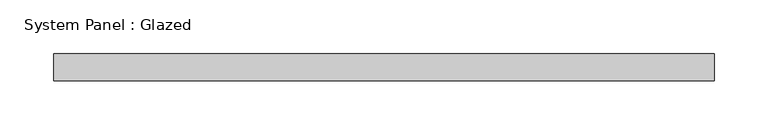
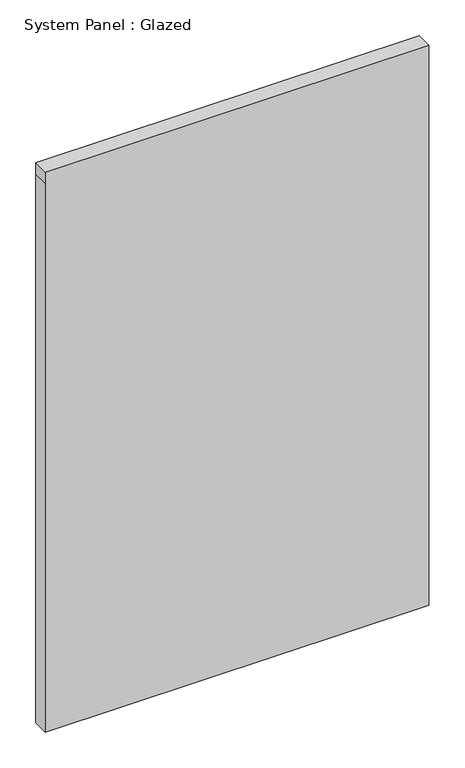
"""IFC4 building model written with IfcOpenShell, lengths in millimetres: plate geometry, System Panel : Glazed."""

from ifc_helpers import new_model, si_unit, frame, origin, place, context, project, spatial, polyline, outline, extrude, source, transform, mapped, element, save


def system_panel_glazed_bb181a04(model_context):
    return source(origin(), model_context, "Body", "SweptSolid", [
        extrude(outline(polyline([(0.0, -307.975), (0.0, 307.975), (931.7680153, 307.975), (950.8180153, 307.975), (950.8180153, -307.975), (931.7680153, -307.975), (0.0, -307.975)])), frame((0.0, 19.05, 0.0), z_axis=(0.0, 1.0, 0.0), x_axis=(0.0, 0.0, 1.0)), (0.0, 0.0, 1.0), 25.4),
    ])


if __name__ == "__main__":
    model = new_model("IFC4")
    model_context = context("Model", 3, world=origin())
    ifc_project = project(units=[si_unit("LENGTHUNIT", "METRE", prefix="MILLI")], contexts=[model_context])
    site = spatial("IfcSite", under=ifc_project)
    building = spatial("IfcBuilding", under=site)
    placement = place(None, origin())
    system_panel_glazed_shape = system_panel_glazed_bb181a04(model_context)
    element("IfcPlate", 1, ObjectType="System Panel : Glazed", at=placement, inside=building, context=model_context, shape_type="MappedRepresentation", body=[
        mapped(system_panel_glazed_shape, transform((0.0, 0.0, 0.0), x_axis=(1.0, 0.0, 0.0), y_axis=(0.0, 1.0, 0.0), z_axis=(0.0, 0.0, 1.0))),
    ])
    save(model, "model.ifc")

# Revit data of these elements
# Type "System Panel : Glazed"
#   Construction Type Id = "GSP4R"
#   Analytic Construction = "1/8 in Pilkington single glazing"
#   Visual Light Transmittance = 0.9
#   Solar Heat Gain Coefficient = 0.86
#   Heat Transfer Coefficient (U) = 1.18115 BTU/(h·ft²·°F)
#   Define Thermal Properties by = 1
# Element 1 (IfcPlate, "System Panel : Glazed")
#   Materials on its faces: "Glass"
# Materials
#   "Glass": class "Glass", colour RGB 0 128 192, transparency 0.75, Description = "Soda Lime Glass", Cost = 0
